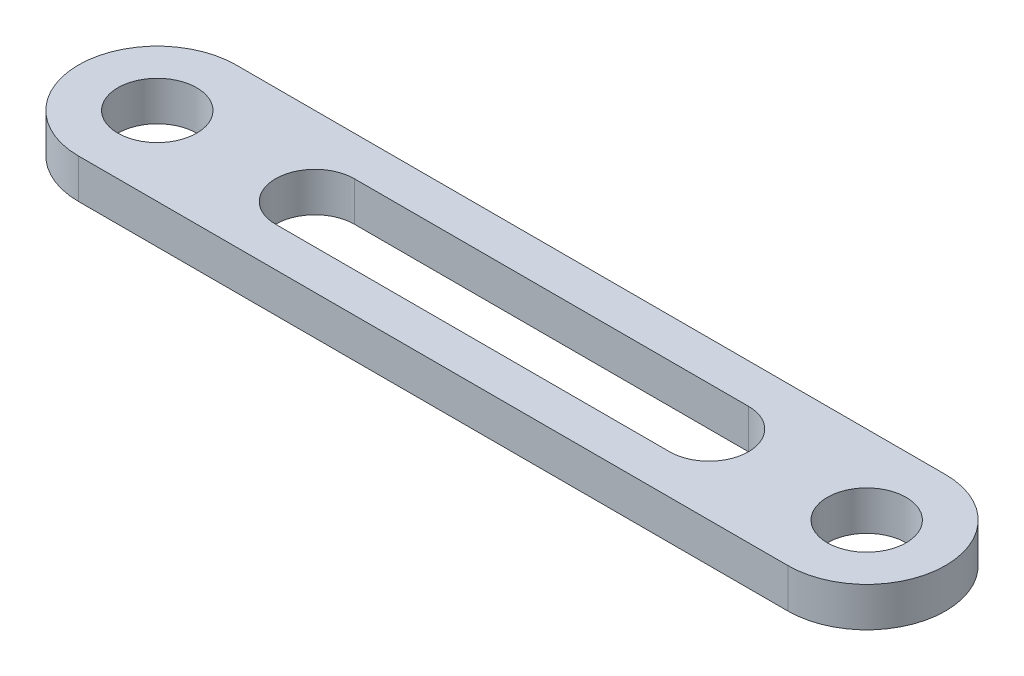
ISO-10303-21;
HEADER;
FILE_DESCRIPTION(('STEP AP214'),'2;1');
FILE_NAME('part.step','',(''),(''),'','','');
FILE_SCHEMA(('AUTOMOTIVE_DESIGN { 1 0 10303 214 1 1 1 1 }'));
ENDSEC;
DATA;
#1=APPLICATION_CONTEXT('core data for automotive mechanical design processes');
#2=APPLICATION_PROTOCOL_DEFINITION('international standard','automotive_design',2000,#1);
#3=PRODUCT_CONTEXT('',#1,'mechanical');
#4=PRODUCT('Part','Part','',(#3));
#5=PRODUCT_RELATED_PRODUCT_CATEGORY('part','',(#4));
#6=PRODUCT_DEFINITION_FORMATION('','',#4);
#7=PRODUCT_DEFINITION_CONTEXT('part definition',#1,'design');
#8=PRODUCT_DEFINITION('design','',#6,#7);
#9=PRODUCT_DEFINITION_SHAPE('','',#8);
#10=(LENGTH_UNIT() NAMED_UNIT(*) SI_UNIT(.MILLI.,.METRE.));
#11=(NAMED_UNIT(*) PLANE_ANGLE_UNIT() SI_UNIT($,.RADIAN.));
#12=(NAMED_UNIT(*) SI_UNIT($,.STERADIAN.) SOLID_ANGLE_UNIT());
#13=UNCERTAINTY_MEASURE_WITH_UNIT(LENGTH_MEASURE(1.E-05),#10,'distance_accuracy_value','');
#14=(GEOMETRIC_REPRESENTATION_CONTEXT(3) GLOBAL_UNCERTAINTY_ASSIGNED_CONTEXT((#13)) GLOBAL_UNIT_ASSIGNED_CONTEXT((#10,
#11,#12)) REPRESENTATION_CONTEXT('',''));
#15=CARTESIAN_POINT('',(0.,0.,0.));
#16=DIRECTION('',(0.,0.,1.));
#17=DIRECTION('',(1.,0.,0.));
#18=AXIS2_PLACEMENT_3D('',#15,#16,#17);
#19=CARTESIAN_POINT('',(-45.,5.,0.));
#20=DIRECTION('',(0.,1.,0.));
#21=DIRECTION('',(0.,0.,1.));
#22=AXIS2_PLACEMENT_3D('',#19,#20,#21);
#23=PLANE('',#22);
#24=CARTESIAN_POINT('',(-45.,5.,0.));
#25=DIRECTION('',(0.,1.,0.));
#26=DIRECTION('',(0.,0.,1.));
#27=AXIS2_PLACEMENT_3D('',#24,#25,#26);
#28=CIRCLE('',#27,5.);
#29=CARTESIAN_POINT('',(-45.,5.,5.));
#30=VERTEX_POINT('',#29);
#31=EDGE_CURVE('E148',#30,#30,#28,.T.);
#32=ORIENTED_EDGE('',*,*,#31,.F.);
#33=EDGE_LOOP('',(#32));
#34=FACE_BOUND('',#33,.T.);
#35=CARTESIAN_POINT('',(-45.,5.,0.));
#36=DIRECTION('',(0.,1.,0.));
#37=DIRECTION('',(0.,0.,1.));
#38=AXIS2_PLACEMENT_3D('',#35,#36,#37);
#39=CIRCLE('',#38,10.);
#40=CARTESIAN_POINT('',(-45.,5.,-10.));
#41=VERTEX_POINT('',#40);
#42=CARTESIAN_POINT('',(-45.,5.,10.));
#43=VERTEX_POINT('',#42);
#44=EDGE_CURVE('E155',#41,#43,#39,.T.);
#45=ORIENTED_EDGE('',*,*,#44,.T.);
#46=DIRECTION('',(1.,0.,0.));
#47=VECTOR('',#46,1.);
#48=CARTESIAN_POINT('',(-45.,5.,10.));
#49=LINE('',#48,#47);
#50=CARTESIAN_POINT('',(45.,5.,9.99999999999998));
#51=VERTEX_POINT('',#50);
#52=EDGE_CURVE('E154',#43,#51,#49,.T.);
#53=ORIENTED_EDGE('',*,*,#52,.T.);
#54=CARTESIAN_POINT('',(45.,5.,0.));
#55=DIRECTION('',(0.,1.,0.));
#56=DIRECTION('',(0.,0.,1.));
#57=AXIS2_PLACEMENT_3D('',#54,#55,#56);
#58=CIRCLE('',#57,10.);
#59=CARTESIAN_POINT('',(45.,5.,-10.));
#60=VERTEX_POINT('',#59);
#61=EDGE_CURVE('E158',#51,#60,#58,.T.);
#62=ORIENTED_EDGE('',*,*,#61,.T.);
#63=DIRECTION('',(-1.,0.,0.));
#64=VECTOR('',#63,1.);
#65=CARTESIAN_POINT('',(-45.,5.,-10.));
#66=LINE('',#65,#64);
#67=EDGE_CURVE('E159',#60,#41,#66,.T.);
#68=ORIENTED_EDGE('',*,*,#67,.T.);
#69=EDGE_LOOP('',(#45,#53,#62,#68));
#70=FACE_BOUND('',#69,.T.);
#71=CARTESIAN_POINT('',(45.,5.,0.));
#72=DIRECTION('',(0.,1.,0.));
#73=DIRECTION('',(0.,0.,1.));
#74=AXIS2_PLACEMENT_3D('',#71,#72,#73);
#75=CIRCLE('',#74,5.);
#76=CARTESIAN_POINT('',(45.,5.,4.99999999999998));
#77=VERTEX_POINT('',#76);
#78=EDGE_CURVE('E138',#77,#77,#75,.T.);
#79=ORIENTED_EDGE('',*,*,#78,.F.);
#80=EDGE_LOOP('',(#79));
#81=FACE_BOUND('',#80,.T.);
#82=DIRECTION('',(1.,0.,0.));
#83=VECTOR('',#82,1.);
#84=CARTESIAN_POINT('',(-25.,5.,5.));
#85=LINE('',#84,#83);
#86=CARTESIAN_POINT('',(-25.,5.,5.));
#87=VERTEX_POINT('',#86);
#88=CARTESIAN_POINT('',(25.,5.,4.99999999999999));
#89=VERTEX_POINT('',#88);
#90=EDGE_CURVE('E115',#87,#89,#85,.T.);
#91=ORIENTED_EDGE('',*,*,#90,.F.);
#92=CARTESIAN_POINT('',(-25.,5.,0.));
#93=DIRECTION('',(0.,1.,0.));
#94=DIRECTION('',(0.,0.,1.));
#95=AXIS2_PLACEMENT_3D('',#92,#93,#94);
#96=CIRCLE('',#95,5.);
#97=CARTESIAN_POINT('',(-25.,5.,-5.));
#98=VERTEX_POINT('',#97);
#99=EDGE_CURVE('E102',#98,#87,#96,.T.);
#100=ORIENTED_EDGE('',*,*,#99,.F.);
#101=DIRECTION('',(-1.,0.,0.));
#102=VECTOR('',#101,1.);
#103=CARTESIAN_POINT('',(-25.,5.,-5.));
#104=LINE('',#103,#102);
#105=CARTESIAN_POINT('',(25.,5.,-5.00000000000001));
#106=VERTEX_POINT('',#105);
#107=EDGE_CURVE('E127',#106,#98,#104,.T.);
#108=ORIENTED_EDGE('',*,*,#107,.F.);
#109=CARTESIAN_POINT('',(25.,5.,0.));
#110=DIRECTION('',(0.,1.,0.));
#111=DIRECTION('',(0.,0.,1.));
#112=AXIS2_PLACEMENT_3D('',#109,#110,#111);
#113=CIRCLE('',#112,5.);
#114=EDGE_CURVE('E121',#89,#106,#113,.T.);
#115=ORIENTED_EDGE('',*,*,#114,.F.);
#116=EDGE_LOOP('',(#91,#100,#108,#115));
#117=FACE_BOUND('',#116,.T.);
#118=ADVANCED_FACE('F39',(#34,#70,#81,#117),#23,.T.);
#119=CARTESIAN_POINT('',(-45.,0.,0.));
#120=DIRECTION('',(0.,1.,0.));
#121=DIRECTION('',(0.,0.,1.));
#122=AXIS2_PLACEMENT_3D('',#119,#120,#121);
#123=PLANE('',#122);
#124=CARTESIAN_POINT('',(45.,0.,0.));
#125=DIRECTION('',(0.,1.,0.));
#126=DIRECTION('',(0.,0.,1.));
#127=AXIS2_PLACEMENT_3D('',#124,#125,#126);
#128=CIRCLE('',#127,5.);
#129=CARTESIAN_POINT('',(45.,0.,4.99999999999998));
#130=VERTEX_POINT('',#129);
#131=EDGE_CURVE('E118',#130,#130,#128,.T.);
#132=ORIENTED_EDGE('',*,*,#131,.T.);
#133=EDGE_LOOP('',(#132));
#134=FACE_BOUND('',#133,.T.);
#135=CARTESIAN_POINT('',(-45.,0.,0.));
#136=DIRECTION('',(0.,1.,0.));
#137=DIRECTION('',(0.,0.,1.));
#138=AXIS2_PLACEMENT_3D('',#135,#136,#137);
#139=CIRCLE('',#138,5.);
#140=CARTESIAN_POINT('',(-45.,0.,5.));
#141=VERTEX_POINT('',#140);
#142=EDGE_CURVE('E141',#141,#141,#139,.T.);
#143=ORIENTED_EDGE('',*,*,#142,.T.);
#144=EDGE_LOOP('',(#143));
#145=FACE_BOUND('',#144,.T.);
#146=CARTESIAN_POINT('',(-45.,0.,0.));
#147=DIRECTION('',(0.,1.,0.));
#148=DIRECTION('',(0.,0.,1.));
#149=AXIS2_PLACEMENT_3D('',#146,#147,#148);
#150=CIRCLE('',#149,10.);
#151=CARTESIAN_POINT('',(-45.,0.,-10.));
#152=VERTEX_POINT('',#151);
#153=CARTESIAN_POINT('',(-45.,0.,10.));
#154=VERTEX_POINT('',#153);
#155=EDGE_CURVE('E149',#152,#154,#150,.T.);
#156=ORIENTED_EDGE('',*,*,#155,.F.);
#157=DIRECTION('',(-1.,0.,0.));
#158=VECTOR('',#157,1.);
#159=CARTESIAN_POINT('',(-45.,0.,-10.));
#160=LINE('',#159,#158);
#161=CARTESIAN_POINT('',(45.,0.,-10.));
#162=VERTEX_POINT('',#161);
#163=EDGE_CURVE('E156',#162,#152,#160,.T.);
#164=ORIENTED_EDGE('',*,*,#163,.F.);
#165=CARTESIAN_POINT('',(45.,0.,0.));
#166=DIRECTION('',(0.,1.,0.));
#167=DIRECTION('',(0.,0.,1.));
#168=AXIS2_PLACEMENT_3D('',#165,#166,#167);
#169=CIRCLE('',#168,10.);
#170=CARTESIAN_POINT('',(45.,0.,9.99999999999998));
#171=VERTEX_POINT('',#170);
#172=EDGE_CURVE('E170',#171,#162,#169,.T.);
#173=ORIENTED_EDGE('',*,*,#172,.F.);
#174=DIRECTION('',(1.,0.,0.));
#175=VECTOR('',#174,1.);
#176=CARTESIAN_POINT('',(-45.,0.,10.));
#177=LINE('',#176,#175);
#178=EDGE_CURVE('E164',#154,#171,#177,.T.);
#179=ORIENTED_EDGE('',*,*,#178,.F.);
#180=EDGE_LOOP('',(#156,#164,#173,#179));
#181=FACE_BOUND('',#180,.T.);
#182=CARTESIAN_POINT('',(-25.,0.,0.));
#183=DIRECTION('',(0.,1.,0.));
#184=DIRECTION('',(0.,0.,1.));
#185=AXIS2_PLACEMENT_3D('',#182,#183,#184);
#186=CIRCLE('',#185,5.);
#187=CARTESIAN_POINT('',(-25.,0.,-5.));
#188=VERTEX_POINT('',#187);
#189=CARTESIAN_POINT('',(-25.,0.,5.));
#190=VERTEX_POINT('',#189);
#191=EDGE_CURVE('E65',#188,#190,#186,.T.);
#192=ORIENTED_EDGE('',*,*,#191,.T.);
#193=DIRECTION('',(1.,0.,0.));
#194=VECTOR('',#193,1.);
#195=CARTESIAN_POINT('',(-25.,0.,5.));
#196=LINE('',#195,#194);
#197=CARTESIAN_POINT('',(25.,0.,4.99999999999999));
#198=VERTEX_POINT('',#197);
#199=EDGE_CURVE('E116',#190,#198,#196,.T.);
#200=ORIENTED_EDGE('',*,*,#199,.T.);
#201=CARTESIAN_POINT('',(25.,0.,0.));
#202=DIRECTION('',(0.,1.,0.));
#203=DIRECTION('',(0.,0.,1.));
#204=AXIS2_PLACEMENT_3D('',#201,#202,#203);
#205=CIRCLE('',#204,5.);
#206=CARTESIAN_POINT('',(25.,0.,-5.00000000000001));
#207=VERTEX_POINT('',#206);
#208=EDGE_CURVE('E135',#198,#207,#205,.T.);
#209=ORIENTED_EDGE('',*,*,#208,.T.);
#210=DIRECTION('',(-1.,0.,0.));
#211=VECTOR('',#210,1.);
#212=CARTESIAN_POINT('',(-25.,0.,-5.));
#213=LINE('',#212,#211);
#214=EDGE_CURVE('E114',#207,#188,#213,.T.);
#215=ORIENTED_EDGE('',*,*,#214,.T.);
#216=EDGE_LOOP('',(#192,#200,#209,#215));
#217=FACE_BOUND('',#216,.T.);
#218=ADVANCED_FACE('F183',(#134,#145,#181,#217),#123,.F.);
#219=CARTESIAN_POINT('',(-45.,5.,0.));
#220=DIRECTION('',(0.,-1.,0.));
#221=DIRECTION('',(0.,0.,-1.));
#222=AXIS2_PLACEMENT_3D('',#219,#220,#221);
#223=CYLINDRICAL_SURFACE('',#222,10.);
#224=ORIENTED_EDGE('',*,*,#155,.T.);
#225=DIRECTION('',(0.,-1.,0.));
#226=VECTOR('',#225,1.);
#227=CARTESIAN_POINT('',(-45.,5.,10.));
#228=LINE('',#227,#226);
#229=EDGE_CURVE('E11',#43,#154,#228,.T.);
#230=ORIENTED_EDGE('',*,*,#229,.F.);
#231=ORIENTED_EDGE('',*,*,#44,.F.);
#232=DIRECTION('',(0.,-1.,0.));
#233=VECTOR('',#232,1.);
#234=CARTESIAN_POINT('',(-45.,5.,-10.));
#235=LINE('',#234,#233);
#236=EDGE_CURVE('E165',#41,#152,#235,.T.);
#237=ORIENTED_EDGE('',*,*,#236,.T.);
#238=EDGE_LOOP('',(#224,#230,#231,#237));
#239=FACE_BOUND('',#238,.T.);
#240=ADVANCED_FACE('F41',(#239),#223,.T.);
#241=CARTESIAN_POINT('',(-45.,5.,10.));
#242=DIRECTION('',(0.,0.,-1.));
#243=DIRECTION('',(-1.,0.,0.));
#244=AXIS2_PLACEMENT_3D('',#241,#242,#243);
#245=PLANE('',#244);
#246=ORIENTED_EDGE('',*,*,#178,.T.);
#247=DIRECTION('',(0.,-1.,0.));
#248=VECTOR('',#247,1.);
#249=CARTESIAN_POINT('',(45.,5.,9.99999999999998));
#250=LINE('',#249,#248);
#251=EDGE_CURVE('E50',#51,#171,#250,.T.);
#252=ORIENTED_EDGE('',*,*,#251,.F.);
#253=ORIENTED_EDGE('',*,*,#52,.F.);
#254=ORIENTED_EDGE('',*,*,#229,.T.);
#255=EDGE_LOOP('',(#246,#252,#253,#254));
#256=FACE_BOUND('',#255,.T.);
#257=ADVANCED_FACE('F198',(#256),#245,.F.);
#258=CARTESIAN_POINT('',(45.,5.,0.));
#259=DIRECTION('',(0.,-1.,0.));
#260=DIRECTION('',(0.,0.,-1.));
#261=AXIS2_PLACEMENT_3D('',#258,#259,#260);
#262=CYLINDRICAL_SURFACE('',#261,10.);
#263=ORIENTED_EDGE('',*,*,#172,.T.);
#264=DIRECTION('',(0.,-1.,0.));
#265=VECTOR('',#264,1.);
#266=CARTESIAN_POINT('',(45.,5.,-10.));
#267=LINE('',#266,#265);
#268=EDGE_CURVE('E175',#60,#162,#267,.T.);
#269=ORIENTED_EDGE('',*,*,#268,.F.);
#270=ORIENTED_EDGE('',*,*,#61,.F.);
#271=ORIENTED_EDGE('',*,*,#251,.T.);
#272=EDGE_LOOP('',(#263,#269,#270,#271));
#273=FACE_BOUND('',#272,.T.);
#274=ADVANCED_FACE('F176',(#273),#262,.T.);
#275=CARTESIAN_POINT('',(-45.,5.,-10.));
#276=DIRECTION('',(0.,0.,1.));
#277=DIRECTION('',(1.,0.,0.));
#278=AXIS2_PLACEMENT_3D('',#275,#276,#277);
#279=PLANE('',#278);
#280=ORIENTED_EDGE('',*,*,#163,.T.);
#281=ORIENTED_EDGE('',*,*,#236,.F.);
#282=ORIENTED_EDGE('',*,*,#67,.F.);
#283=ORIENTED_EDGE('',*,*,#268,.T.);
#284=EDGE_LOOP('',(#280,#281,#282,#283));
#285=FACE_BOUND('',#284,.T.);
#286=ADVANCED_FACE('F186',(#285),#279,.F.);
#287=CARTESIAN_POINT('',(-45.,5.,0.));
#288=DIRECTION('',(0.,-1.,0.));
#289=DIRECTION('',(0.,0.,-1.));
#290=AXIS2_PLACEMENT_3D('',#287,#288,#289);
#291=CYLINDRICAL_SURFACE('',#290,5.);
#292=ORIENTED_EDGE('',*,*,#31,.T.);
#293=EDGE_LOOP('',(#292));
#294=FACE_BOUND('',#293,.T.);
#295=ORIENTED_EDGE('',*,*,#142,.F.);
#296=EDGE_LOOP('',(#295));
#297=FACE_BOUND('',#296,.T.);
#298=ADVANCED_FACE('F213',(#294,#297),#291,.F.);
#299=CARTESIAN_POINT('',(45.,5.,0.));
#300=DIRECTION('',(0.,-1.,0.));
#301=DIRECTION('',(0.,0.,-1.));
#302=AXIS2_PLACEMENT_3D('',#299,#300,#301);
#303=CYLINDRICAL_SURFACE('',#302,5.);
#304=ORIENTED_EDGE('',*,*,#78,.T.);
#305=EDGE_LOOP('',(#304));
#306=FACE_BOUND('',#305,.T.);
#307=ORIENTED_EDGE('',*,*,#131,.F.);
#308=EDGE_LOOP('',(#307));
#309=FACE_BOUND('',#308,.T.);
#310=ADVANCED_FACE('F219',(#306,#309),#303,.F.);
#311=CARTESIAN_POINT('',(-25.,5.,0.));
#312=DIRECTION('',(0.,-1.,0.));
#313=DIRECTION('',(0.,0.,-1.));
#314=AXIS2_PLACEMENT_3D('',#311,#312,#313);
#315=CYLINDRICAL_SURFACE('',#314,5.);
#316=ORIENTED_EDGE('',*,*,#191,.F.);
#317=DIRECTION('',(0.,-1.,0.));
#318=VECTOR('',#317,1.);
#319=CARTESIAN_POINT('',(-25.,5.,-5.));
#320=LINE('',#319,#318);
#321=EDGE_CURVE('E107',#98,#188,#320,.T.);
#322=ORIENTED_EDGE('',*,*,#321,.F.);
#323=ORIENTED_EDGE('',*,*,#99,.T.);
#324=DIRECTION('',(0.,-1.,0.));
#325=VECTOR('',#324,1.);
#326=CARTESIAN_POINT('',(-25.,5.,5.));
#327=LINE('',#326,#325);
#328=EDGE_CURVE('E110',#87,#190,#327,.T.);
#329=ORIENTED_EDGE('',*,*,#328,.T.);
#330=EDGE_LOOP('',(#316,#322,#323,#329));
#331=FACE_BOUND('',#330,.T.);
#332=ADVANCED_FACE('F106',(#331),#315,.F.);
#333=CARTESIAN_POINT('',(-25.,5.,5.));
#334=DIRECTION('',(0.,0.,-1.));
#335=DIRECTION('',(-1.,0.,0.));
#336=AXIS2_PLACEMENT_3D('',#333,#334,#335);
#337=PLANE('',#336);
#338=ORIENTED_EDGE('',*,*,#199,.F.);
#339=ORIENTED_EDGE('',*,*,#328,.F.);
#340=ORIENTED_EDGE('',*,*,#90,.T.);
#341=DIRECTION('',(0.,-1.,0.));
#342=VECTOR('',#341,1.);
#343=CARTESIAN_POINT('',(25.,5.,4.99999999999999));
#344=LINE('',#343,#342);
#345=EDGE_CURVE('E122',#89,#198,#344,.T.);
#346=ORIENTED_EDGE('',*,*,#345,.T.);
#347=EDGE_LOOP('',(#338,#339,#340,#346));
#348=FACE_BOUND('',#347,.T.);
#349=ADVANCED_FACE('F117',(#348),#337,.T.);
#350=CARTESIAN_POINT('',(25.,5.,0.));
#351=DIRECTION('',(0.,-1.,0.));
#352=DIRECTION('',(0.,0.,-1.));
#353=AXIS2_PLACEMENT_3D('',#350,#351,#352);
#354=CYLINDRICAL_SURFACE('',#353,5.);
#355=ORIENTED_EDGE('',*,*,#208,.F.);
#356=ORIENTED_EDGE('',*,*,#345,.F.);
#357=ORIENTED_EDGE('',*,*,#114,.T.);
#358=DIRECTION('',(0.,-1.,0.));
#359=VECTOR('',#358,1.);
#360=CARTESIAN_POINT('',(25.,5.,-5.00000000000001));
#361=LINE('',#360,#359);
#362=EDGE_CURVE('E53',#106,#207,#361,.T.);
#363=ORIENTED_EDGE('',*,*,#362,.T.);
#364=EDGE_LOOP('',(#355,#356,#357,#363));
#365=FACE_BOUND('',#364,.T.);
#366=ADVANCED_FACE('F240',(#365),#354,.F.);
#367=CARTESIAN_POINT('',(-25.,5.,-5.));
#368=DIRECTION('',(0.,0.,1.));
#369=DIRECTION('',(1.,0.,0.));
#370=AXIS2_PLACEMENT_3D('',#367,#368,#369);
#371=PLANE('',#370);
#372=ORIENTED_EDGE('',*,*,#214,.F.);
#373=ORIENTED_EDGE('',*,*,#362,.F.);
#374=ORIENTED_EDGE('',*,*,#107,.T.);
#375=ORIENTED_EDGE('',*,*,#321,.T.);
#376=EDGE_LOOP('',(#372,#373,#374,#375));
#377=FACE_BOUND('',#376,.T.);
#378=ADVANCED_FACE('F238',(#377),#371,.T.);
#379=CLOSED_SHELL('',(#118,#218,#240,#257,#274,#286,#298,#310,#332,#349,#366,#378));
#380=MANIFOLD_SOLID_BREP('B2',#379);
#381=ADVANCED_BREP_SHAPE_REPRESENTATION('',(#18,#380),#14);
#382=SHAPE_DEFINITION_REPRESENTATION(#9,#381);
ENDSEC;
END-ISO-10303-21;
